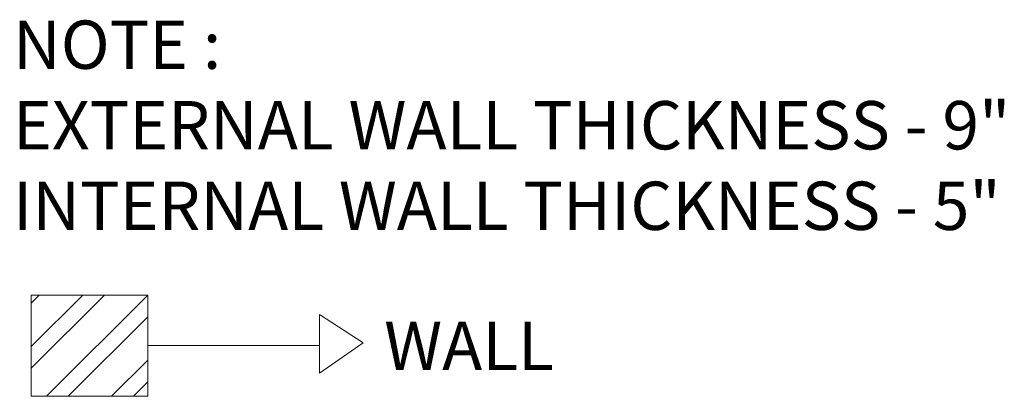
# Model space of a CAD drawing. Units: inches. Extents: x 683 to 1274, y 1901 to 2385.
# Tile 5 of 5: x 1070 to 1274, y 2106 to 2184. Entities that reach past the tile are written whole.
import ezdxf

# ---------------------------------------------------------------- set-up
doc = ezdxf.new("R2010")
doc.units = ezdxf.units.IN
for name, color, linetype, lineweight in [('A-ANNO-SYMB', 1, 'Continuous', 18), ('A-WALL-PATT', 8, 'Continuous', 13), ('TEXT', 1, 'Continuous', 25)]:
    doc.layers.add(name, color=color, linetype=linetype, lineweight=lineweight)
doc.styles.get("Standard").update_dxf_attribs({"font": 'arial.ttf'})

msp = doc.modelspace()

# ---------------------------------------------------------------- hatches: boundary and pattern name
at = {"layer": 'A-WALL-PATT'}
h = msp.add_hatch(dxfattribs=at)
h.set_pattern_fill('ANSI32', color=256)
h.set_pattern_definition([(45, (1.143, 128.543), (-6.735192, 6.735192), []), (45, (5.633, 128.543), (-6.735192, 6.735192), [])])
h.paths.add_polyline_path([(1096.63, 2126.56), (1072.53, 2126.56), (1072.53, 2105.6), (1096.63, 2105.6)])

# ---------------------------------------------------------------- linework, layer by layer
at = {"layer": 'A-ANNO-SYMB'}
for p, q in [((1132.14, 2122.5), (1132.14, 2110.39)), ((1141.13, 2116.64), (1132.14, 2122.5)), ((1096.63, 2116.08), (1132.14, 2116.08)), ((1132.14, 2110.39), (1141.13, 2116.64))]:
    msp.add_line(p, q, dxfattribs=at)
msp.add_lwpolyline([(1072.53, 2126.56), (1096.63, 2126.56), (1096.63, 2105.6), (1072.53, 2105.6)], close=True, dxfattribs=at)

# ---------------------------------------------------------------- texts
at = {"layer": 'TEXT', "char_height": 10, "attachment_point": 1}
for s, width, insert in [('{NOTE :\\PEXTERNAL WALL THICKNESS - 9"\\PINTERNAL WALL THICKNESS - 5"}', 253.0673, (1068.77, 2183.36)), ('WALL ', 37.9223, (1145.49, 2121.03))]:
    msp.add_mtext_dynamic_manual_height_columns(s, width=width, gutter_width=12.5, heights=[0], dxfattribs=dict(at, insert=insert))

doc.saveas('drawing.dxf')
